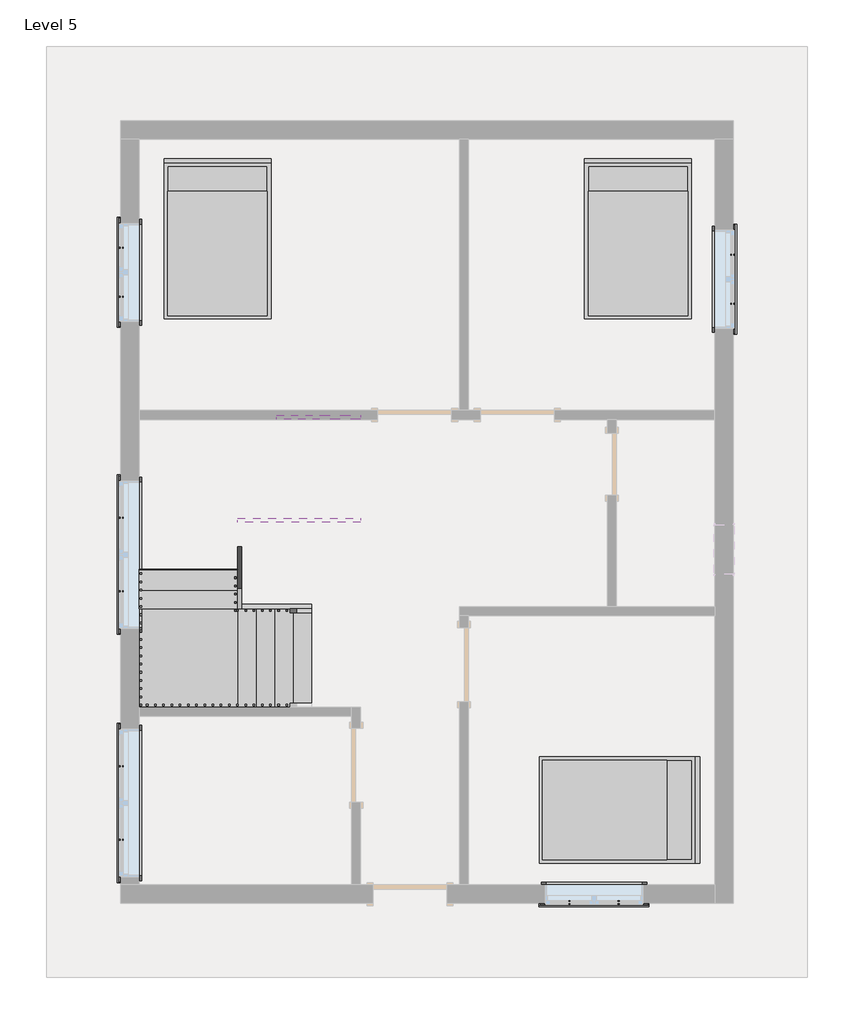
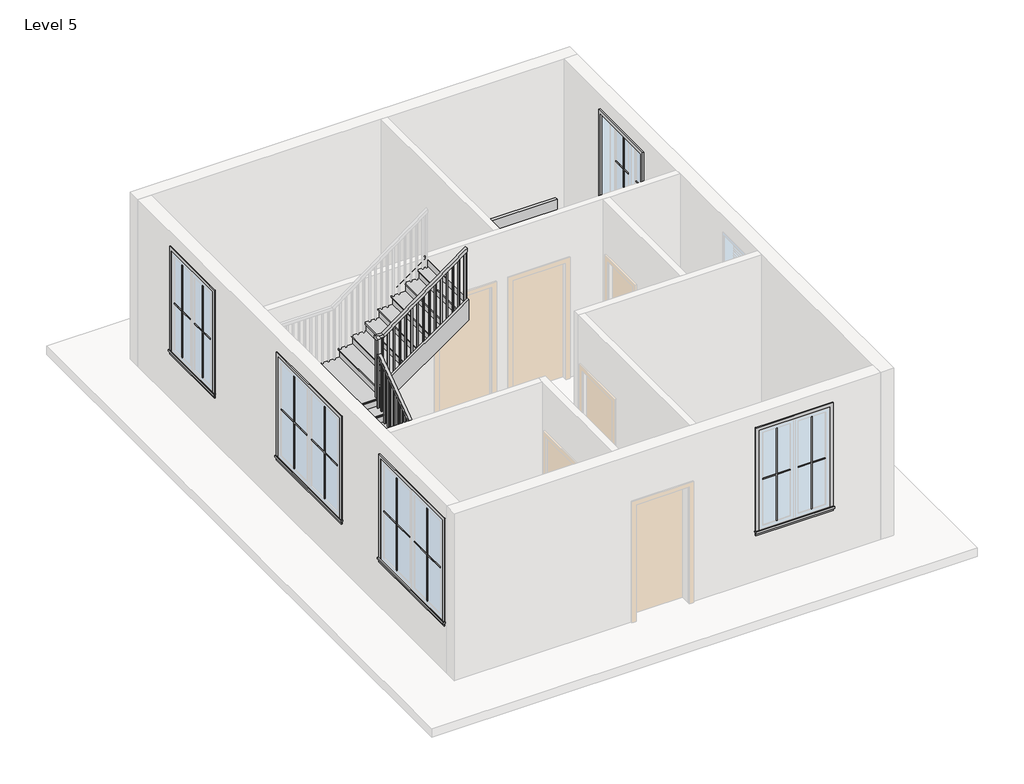
# One storey, part 3 of 3: 20 proxies, 5 members, 3 furniture elements, 1 railing, 1 stair flight.
"""IFC4 building model written with IfcOpenShell, lengths in millimetres."""

from ifc_helpers import new_model, si_unit, frame, origin, place, context, project, spatial, polyline, outline, extrude, faceted_brep, transform, mapped, element, save
from components import muntin_pattern_2x2_muntin_pattern_2x2_0a037076, muntin_pattern_2x2_muntin_pattern_2x2_e6f69628, muntin_pattern_2x2_muntin_pattern_2x2_2b4d9f72, muntin_pattern_2x2_muntin_pattern_2x2_ef995ed3, trim_window_exterior_flat_with_sill_b601e94a, trim_window_exterior_flat_with_sill_b7e4d11c, trim_window_interior_flat_picture_frame_bfefb25c, trim_window_interior_flat_picture_frame_936b8d2a, bed_17739_bed_17739_15c61121, stair_flight_d9589ae6

model = new_model("IFC4")

# Units and contexts
model_context = context("Model", 3, world=origin())
ifc_project = project(units=[si_unit("LENGTHUNIT", "METRE", prefix="MILLI")], contexts=[model_context])

# Site, building, storey
site = spatial("IfcSite", under=ifc_project)
building = spatial("IfcBuilding", under=site)
storey = spatial("IfcBuildingStorey", under=building, Name="Level 5", Elevation=12649.2)

# Proxies
placement = place(None, origin())
muntin_pattern_2x2_muntin_pattern_2x2_shape = muntin_pattern_2x2_muntin_pattern_2x2_0a037076(model_context)
element("IfcBuildingElementProxy", 1, Name="Muntin Pattern_2x2 : Muntin Pattern_2x2", ObjectType="Muntin Pattern_2x2 : Muntin Pattern_2x2", at=placement, inside=storey, context=model_context, shape_type="MappedRepresentation", body=[
    mapped(muntin_pattern_2x2_muntin_pattern_2x2_shape, transform((-5035.7855391, -4380.9248761, 13633.45), x_axis=(0.0, 1.0, 0.0), y_axis=(-1.0, 0.0, 0.0), z_axis=(0.0, 0.0, 1.0))),
])
element("IfcBuildingElementProxy", 2, Name="Muntin Pattern_2x2 : Muntin Pattern_2x2", ObjectType="Muntin Pattern_2x2 : Muntin Pattern_2x2", at=placement, inside=storey, context=model_context, shape_type="MappedRepresentation", body=[
    mapped(muntin_pattern_2x2_muntin_pattern_2x2_shape, transform((-5035.7855391, -1310.6998761, 13633.45), x_axis=(0.0, 1.0, 0.0), y_axis=(-1.0, 0.0, 0.0), z_axis=(0.0, 0.0, 1.0))),
])
muntin_pattern_2x2_muntin_pattern_2x2_2_shape = muntin_pattern_2x2_muntin_pattern_2x2_e6f69628(model_context)
element("IfcBuildingElementProxy", 3, Name="Muntin Pattern_2x2 : Muntin Pattern_2x2", ObjectType="Muntin Pattern_2x2 : Muntin Pattern_2x2", at=placement, inside=storey, context=model_context, shape_type="MappedRepresentation", body=[
    mapped(muntin_pattern_2x2_muntin_pattern_2x2_2_shape, transform((-5035.7855391, -3469.6998761, 13633.45), x_axis=(0.0, -1.0, 0.0), y_axis=(1.0, 0.0, 0.0), z_axis=(0.0, 0.0, 1.0))),
])
element("IfcBuildingElementProxy", 4, Name="Muntin Pattern_2x2 : Muntin Pattern_2x2", ObjectType="Muntin Pattern_2x2 : Muntin Pattern_2x2", at=placement, inside=storey, context=model_context, shape_type="MappedRepresentation", body=[
    mapped(muntin_pattern_2x2_muntin_pattern_2x2_2_shape, transform((-5035.7855391, -399.4748761, 13633.45), x_axis=(0.0, -1.0, 0.0), y_axis=(1.0, 0.0, 0.0), z_axis=(0.0, 0.0, 1.0))),
])
muntin_pattern_2x2_muntin_pattern_2x2_3_shape = muntin_pattern_2x2_muntin_pattern_2x2_2b4d9f72(model_context)
element("IfcBuildingElementProxy", 5, Name="Muntin Pattern_2x2 : Muntin Pattern_2x2", ObjectType="Muntin Pattern_2x2 : Muntin Pattern_2x2", at=placement, inside=storey, context=model_context, shape_type="MappedRepresentation", body=[
    mapped(muntin_pattern_2x2_muntin_pattern_2x2_3_shape, transform((1115.7769609, -5157.2123761, 13633.45), x_axis=(-1.0, 0.0, 0.0), y_axis=(0.0, -1.0, 0.0), z_axis=(0.0, 0.0, 1.0))),
])
element("IfcBuildingElementProxy", 6, Name="Muntin Pattern_2x2 : Muntin Pattern_2x2", ObjectType="Muntin Pattern_2x2 : Muntin Pattern_2x2", at=placement, inside=storey, context=model_context, shape_type="MappedRepresentation", body=[
    mapped(muntin_pattern_2x2_muntin_pattern_2x2_3_shape, transform((2527.0644609, 2851.7251239, 13633.45), x_axis=(0.0, -1.0, 0.0), y_axis=(1.0, 0.0, 0.0), z_axis=(0.0, 0.0, 1.0))),
])
element("IfcBuildingElementProxy", 7, Name="Muntin Pattern_2x2 : Muntin Pattern_2x2", ObjectType="Muntin Pattern_2x2 : Muntin Pattern_2x2", at=placement, inside=storey, context=model_context, shape_type="MappedRepresentation", body=[
    mapped(muntin_pattern_2x2_muntin_pattern_2x2_3_shape, transform((-5035.7855391, 2331.0251239, 13633.45), x_axis=(0.0, 1.0, 0.0), y_axis=(-1.0, 0.0, 0.0), z_axis=(0.0, 0.0, 1.0))),
])
muntin_pattern_2x2_muntin_pattern_2x2_4_shape = muntin_pattern_2x2_muntin_pattern_2x2_ef995ed3(model_context)
element("IfcBuildingElementProxy", 8, Name="Muntin Pattern_2x2 : Muntin Pattern_2x2", ObjectType="Muntin Pattern_2x2 : Muntin Pattern_2x2", at=placement, inside=storey, context=model_context, shape_type="MappedRepresentation", body=[
    mapped(muntin_pattern_2x2_muntin_pattern_2x2_4_shape, transform((509.3519609, -5157.2123761, 13633.45), x_axis=(1.0, 0.0, 0.0), y_axis=(0.0, 1.0, 0.0), z_axis=(0.0, 0.0, 1.0))),
])
element("IfcBuildingElementProxy", 9, Name="Muntin Pattern_2x2 : Muntin Pattern_2x2", ObjectType="Muntin Pattern_2x2 : Muntin Pattern_2x2", at=placement, inside=storey, context=model_context, shape_type="MappedRepresentation", body=[
    mapped(muntin_pattern_2x2_muntin_pattern_2x2_4_shape, transform((2527.0644609, 2245.3001239, 13633.45), x_axis=(0.0, 1.0, 0.0), y_axis=(-1.0, 0.0, 0.0), z_axis=(0.0, 0.0, 1.0))),
])
element("IfcBuildingElementProxy", 10, Name="Muntin Pattern_2x2 : Muntin Pattern_2x2", ObjectType="Muntin Pattern_2x2 : Muntin Pattern_2x2", at=placement, inside=storey, context=model_context, shape_type="MappedRepresentation", body=[
    mapped(muntin_pattern_2x2_muntin_pattern_2x2_4_shape, transform((-5035.7855391, 2937.4501239, 13633.45), x_axis=(0.0, -1.0, 0.0), y_axis=(1.0, 0.0, 0.0), z_axis=(0.0, 0.0, 1.0))),
])
trim_window_exterior_flat_with_sill_shape = trim_window_exterior_flat_with_sill_b601e94a(model_context)
element("IfcBuildingElementProxy", 11, Name="Trim-Window-Exterior-Flat : with Sill", ObjectType="Trim-Window-Exterior-Flat : with Sill", at=placement, inside=storey, context=model_context, shape_type="MappedRepresentation", body=[
    mapped(trim_window_exterior_flat_with_sill_shape, transform((-5045.3105391, -3925.3123761, 15392.4), x_axis=(0.0, -1.0, 0.0), y_axis=(0.0, 0.0, 1.0), z_axis=(-1.0, 0.0, 0.0))),
])
element("IfcBuildingElementProxy", 12, Name="Trim-Window-Exterior-Flat : with Sill", ObjectType="Trim-Window-Exterior-Flat : with Sill", at=placement, inside=storey, context=model_context, shape_type="MappedRepresentation", body=[
    mapped(trim_window_exterior_flat_with_sill_shape, transform((-5045.3105391, -855.0873761, 15392.4), x_axis=(0.0, -1.0, 0.0), y_axis=(0.0, 0.0, 1.0), z_axis=(-1.0, 0.0, 0.0))),
])
trim_window_exterior_flat_with_sill_2_shape = trim_window_exterior_flat_with_sill_b7e4d11c(model_context)
element("IfcBuildingElementProxy", 13, Name="Trim-Window-Exterior-Flat : with Sill", ObjectType="Trim-Window-Exterior-Flat : with Sill", at=placement, inside=storey, context=model_context, shape_type="MappedRepresentation", body=[
    mapped(trim_window_exterior_flat_with_sill_2_shape, transform((812.5644609, -5166.7373761, 15392.4), x_axis=(1.0, 0.0, 0.0), y_axis=(0.0, 0.0, 1.0), z_axis=(0.0, -1.0, 0.0))),
])
element("IfcBuildingElementProxy", 14, Name="Trim-Window-Exterior-Flat : with Sill", ObjectType="Trim-Window-Exterior-Flat : with Sill", at=placement, inside=storey, context=model_context, shape_type="MappedRepresentation", body=[
    mapped(trim_window_exterior_flat_with_sill_2_shape, transform((2536.5894609, 2548.5126239, 15392.4), x_axis=(0.0, 1.0, 0.0), y_axis=(0.0, 0.0, 1.0), z_axis=(1.0, 0.0, 0.0))),
])
element("IfcBuildingElementProxy", 15, Name="Trim-Window-Exterior-Flat : with Sill", ObjectType="Trim-Window-Exterior-Flat : with Sill", at=placement, inside=storey, context=model_context, shape_type="MappedRepresentation", body=[
    mapped(trim_window_exterior_flat_with_sill_2_shape, transform((-5045.3105391, 2634.2376239, 15392.4), x_axis=(0.0, -1.0, 0.0), y_axis=(0.0, 0.0, 1.0), z_axis=(-1.0, 0.0, 0.0))),
])
trim_window_interior_flat_picture_frame_shape = trim_window_interior_flat_picture_frame_bfefb25c(model_context)
element("IfcBuildingElementProxy", 16, Name="Trim-Window-Interior-Flat : Picture Frame", ObjectType="Trim-Window-Interior-Flat : Picture Frame", at=placement, inside=storey, context=model_context, shape_type="MappedRepresentation", body=[
    mapped(trim_window_interior_flat_picture_frame_shape, transform((-4816.7105391, -3925.3123761, 15392.4), x_axis=(0.0, 1.0, 0.0), y_axis=(0.0, 0.0, 1.0), z_axis=(1.0, 0.0, 0.0))),
])
element("IfcBuildingElementProxy", 17, Name="Trim-Window-Interior-Flat : Picture Frame", ObjectType="Trim-Window-Interior-Flat : Picture Frame", at=placement, inside=storey, context=model_context, shape_type="MappedRepresentation", body=[
    mapped(trim_window_interior_flat_picture_frame_shape, transform((-4816.7105391, -855.0873761, 15392.4), x_axis=(0.0, 1.0, 0.0), y_axis=(0.0, 0.0, 1.0), z_axis=(1.0, 0.0, 0.0))),
])
trim_window_interior_flat_picture_frame_2_shape = trim_window_interior_flat_picture_frame_936b8d2a(model_context)
element("IfcBuildingElementProxy", 18, Name="Trim-Window-Interior-Flat : Picture Frame", ObjectType="Trim-Window-Interior-Flat : Picture Frame", at=placement, inside=storey, context=model_context, shape_type="MappedRepresentation", body=[
    mapped(trim_window_interior_flat_picture_frame_2_shape, transform((812.5644609, -4938.1373761, 15392.4), x_axis=(-1.0, 0.0, 0.0), y_axis=(0.0, 0.0, 1.0), z_axis=(0.0, 1.0, 0.0))),
])
element("IfcBuildingElementProxy", 19, Name="Trim-Window-Interior-Flat : Picture Frame", ObjectType="Trim-Window-Interior-Flat : Picture Frame", at=placement, inside=storey, context=model_context, shape_type="MappedRepresentation", body=[
    mapped(trim_window_interior_flat_picture_frame_2_shape, transform((2307.9894609, 2548.5126239, 15392.4), x_axis=(0.0, -1.0, 0.0), y_axis=(0.0, 0.0, 1.0), z_axis=(-1.0, 0.0, 0.0))),
])
element("IfcBuildingElementProxy", 20, Name="Trim-Window-Interior-Flat : Picture Frame", ObjectType="Trim-Window-Interior-Flat : Picture Frame", at=placement, inside=storey, context=model_context, shape_type="MappedRepresentation", body=[
    mapped(trim_window_interior_flat_picture_frame_2_shape, transform((-4816.7105391, 2634.2376239, 15392.4), x_axis=(0.0, 1.0, 0.0), y_axis=(0.0, 0.0, 1.0), z_axis=(1.0, 0.0, 0.0))),
])

# Furniture
bed_17739_bed_17739_shape = bed_17739_bed_17739_15c61121(model_context)
element("IfcFurniture", 21, ObjectType="Bed_17739 : Bed_17739", at=placement, inside=storey, context=model_context, shape_type="MappedRepresentation", body=[
    mapped(bed_17739_bed_17739_shape, transform((-3845.1605391, 3024.7626239, 12649.2), x_axis=(1.0, 0.0, 0.0), y_axis=(0.0, 1.0, 0.0), z_axis=(0.0, 0.0, 1.0))),
])
element("IfcFurniture", 22, ObjectType="Bed_17739 : Bed_17739", at=placement, inside=storey, context=model_context, shape_type="MappedRepresentation", body=[
    mapped(bed_17739_bed_17739_shape, transform((1355.4894609, 3024.7626239, 12649.2), x_axis=(1.0, 0.0, 0.0), y_axis=(0.0, 1.0, 0.0), z_axis=(0.0, 0.0, 1.0))),
])
element("IfcFurniture", 23, ObjectType="Bed_17739 : Bed_17739", at=placement, inside=storey, context=model_context, shape_type="MappedRepresentation", body=[
    mapped(bed_17739_bed_17739_shape, transform((1101.4894609, -4011.0373761, 12649.2), x_axis=(0.0, -1.0, 0.0), y_axis=(1.0, 0.0, 0.0), z_axis=(0.0, 0.0, 1.0))),
])

# Members
element("IfcMember", 24, ObjectType="Stringer - 2\" Width", at=placement, inside=storey, context=model_context, shape_type="SweptSolid", body=[
    extrude(outline(polyline([(12649.2, -2683.1105391), (12799.7087903, -2683.1105391), (12799.7087903, -3112.2707489), (12649.2, -2897.7957228), (12649.2, -2683.1105391)])), frame((0.0, -2791.8373761, 0.0), z_axis=(0.0, 1.0, 0.0), x_axis=(0.0, 0.0, 1.0)), (0.0, 0.0, 1.0), 50.8),
])
element("IfcMember", 25, ObjectType="Stringer - 2\" Width", at=placement, inside=storey, context=model_context, shape_type="SweptSolid", body=[
    extrude(outline(polyline([(14976.6856495, -2580.7583047), (15332.6489938, -2073.5105391), (15705.0117181, -2073.5105391), (14976.6856495, -3111.3751869), (14976.6856495, -2580.7583047)])), frame((0.0, 814.9626239, 0.0), z_axis=(0.0, 1.0, 0.0), x_axis=(0.0, 0.0, 1.0)), (0.0, 0.0, 1.0), 50.8),
])
element("IfcMember", 26, ObjectType="Stringer - 2\" Width", at=placement, inside=storey, context=model_context, shape_type="SweptSolid", body=[
    extrude(outline(polyline([(12649.2, -2683.1105391), (12870.906455, -2683.1105391), (13476.9415427, -3546.7105391), (13104.5788184, -3546.7105391), (12649.2, -2897.7957228), (12649.2, -2683.1105391)])), frame((0.0, -1521.8373761, 0.0), z_axis=(0.0, 1.0, 0.0), x_axis=(0.0, 0.0, 1.0)), (0.0, 0.0, 1.0), 50.8),
])
element("IfcMember", 27, ObjectType="Stringer - 2\" Width", at=placement, inside=storey, context=model_context, shape_type="SweptSolid", body=[
    extrude(outline(polyline([(-1521.8373761, 13299.5564629), (-1521.8373761, 13674.7327137), (-455.0373761, 14440.3786467), (-455.0373761, 14065.2023959), (-1521.8373761, 13299.5564629)])), frame((-3597.5105391, 0.0, 0.0), z_axis=(1.0, 0.0, 0.0), x_axis=(0.0, 1.0, 0.0)), (0.0, 0.0, 1.0), 50.8),
])
element("IfcMember", 28, ObjectType="Stringer - 2\" Width", at=placement, inside=storey, context=model_context, shape_type="SweptSolid", body=[
    extrude(outline(polyline([(14635.5380339, -3597.5105391), (14263.1753096, -3597.5105391), (15332.6489938, -2073.5105391), (15705.0117181, -2073.5105391), (14635.5380339, -3597.5105391)])), frame((0.0, -455.0373761, 0.0), z_axis=(0.0, 1.0, 0.0), x_axis=(0.0, 0.0, 1.0)), (0.0, 0.0, 1.0), 50.8),
])

# Railing
element("IfcRailing", 29, ObjectType="Handrail - Rectangular", at=placement, inside=storey, context=model_context, shape_type="SolidModel", body=[
    faceted_brep([(-2683.1105391, -1572.6373761, 13724.0210526), (-2683.1105391, -1572.6373761, 13661.9605986), (-2683.1105391, -1521.8373761, 13661.9605986), (-2683.1105391, -1521.8373761, 13724.0210526), (-3521.3105391, -1572.6373761, 14312.2315789), (-3572.1105391, -1572.6373761, 14285.8202477), (-3572.1105391, -1521.8373761, 14285.8202477), (-3521.3105391, -1521.8373761, 14312.2315789), (-3521.3105391, -1572.6373761, 14580.815311), (-3572.1105391, -1572.6373761, 14530.015311), (-3572.1105391, -1521.8373761, 14530.015311), (-3521.3105391, -1521.8373761, 14580.815311), (-3648.3105391, -1572.6373761, 14580.815311), (-3648.3105391, -1572.6373761, 14530.015311), (-3597.5105391, -1521.8373761, 14530.015311), (-3597.5105391, -1521.8373761, 14580.815311), (-3648.3105391, -1445.6373761, 14580.815311), (-3648.3105391, -1429.2944467, 14530.015311), (-3597.5105391, -1429.2944467, 14530.015311), (-3597.5105391, -1445.6373761, 14580.815311), (-3648.3105391, -480.4373761, 15273.5425837), (-3648.3105391, -429.6373761, 15247.4725387), (-3597.5105391, -429.6373761, 15247.4725387), (-3597.5105391, -480.4373761, 15273.5425837), (-3648.3105391, -480.4373761, 15544.8), (-3648.3105391, -429.6373761, 15494.0), (-3597.5105391, -429.6373761, 15494.0), (-3597.5105391, -480.4373761, 15544.8), (-3648.3105391, -353.4373761, 15544.8), (-3648.3105391, -353.4373761, 15494.0), (-3597.5105391, -404.2373761, 15494.0), (-3597.5105391, -404.2373761, 15544.8), (-3521.3105391, -353.4373761, 15544.8), (-3504.6160355, -353.4373761, 15494.0), (-3504.6160355, -404.2373761, 15494.0), (-3521.3105391, -404.2373761, 15544.8), (-2073.5105391, -353.4373761, 16611.6), (-2073.5105391, -404.2373761, 16611.6), (-2073.5105391, -404.2373761, 16548.4987868), (-2073.5105391, -353.4373761, 16548.4987868)], [[[0, 1, 2, 3]], [[1, 0, 4, 5]], [[2, 1, 5, 6]], [[3, 2, 6, 7]], [[0, 3, 7, 4]], [[5, 4, 8, 9]], [[6, 5, 9, 10]], [[7, 6, 10, 11]], [[4, 7, 11, 8]], [[9, 8, 12, 13]], [[10, 9, 13, 14]], [[11, 10, 14, 15]], [[8, 11, 15, 12]], [[13, 12, 16, 17]], [[14, 13, 17, 18]], [[15, 14, 18, 19]], [[12, 15, 19, 16]], [[17, 16, 20, 21]], [[18, 17, 21, 22]], [[19, 18, 22, 23]], [[16, 19, 23, 20]], [[21, 20, 24, 25]], [[22, 21, 25, 26]], [[23, 22, 26, 27]], [[20, 23, 27, 24]], [[25, 24, 28, 29]], [[26, 25, 29, 30]], [[27, 26, 30, 31]], [[24, 27, 31, 28]], [[29, 28, 32, 33]], [[30, 29, 33, 34]], [[31, 30, 34, 35]], [[28, 31, 35, 32]], [[36, 37, 38, 39]], [[33, 32, 36, 39]], [[34, 33, 39, 38]], [[35, 34, 38, 37]], [[32, 35, 37, 36]]]),
    extrude(outline(polyline([(16536.8014184, -2089.3855391), (16522.7645763, -2108.4355391), (15536.7789474, -2108.4355391), (15536.7789474, -2089.3855391), (16536.8014184, -2089.3855391)])), frame((0.0, -388.3623761, 0.0), z_axis=(0.0, 1.0, 0.0), x_axis=(0.0, 0.0, 1.0)), (0.0, 0.0, 1.0), 19.05),
    extrude(outline(polyline([(16461.9382605, -2190.9855391), (16447.9014184, -2210.0355391), (15536.7789474, -2210.0355391), (15536.7789474, -2190.9855391), (16461.9382605, -2190.9855391)])), frame((0.0, -388.3623761, 0.0), z_axis=(0.0, 1.0, 0.0), x_axis=(0.0, 0.0, 1.0)), (0.0, 0.0, 1.0), 19.05),
    extrude(outline(polyline([(16387.0751026, -2292.5855391), (16373.0382605, -2311.6355391), (15376.3578947, -2311.6355391), (15376.3578947, -2292.5855391), (16387.0751026, -2292.5855391)])), frame((0.0, -388.3623761, 0.0), z_axis=(0.0, 1.0, 0.0), x_axis=(0.0, 0.0, 1.0)), (0.0, 0.0, 1.0), 19.05),
    extrude(outline(polyline([(16312.2119447, -2394.1855391), (16298.1751026, -2413.2355391), (15376.3578947, -2413.2355391), (15376.3578947, -2394.1855391), (16312.2119447, -2394.1855391)])), frame((0.0, -388.3623761, 0.0), z_axis=(0.0, 1.0, 0.0), x_axis=(0.0, 0.0, 1.0)), (0.0, 0.0, 1.0), 19.05),
    extrude(outline(polyline([(16237.3487868, -2495.7855391), (16223.3119447, -2514.8355391), (15215.9368421, -2514.8355391), (15215.9368421, -2495.7855391), (16237.3487868, -2495.7855391)])), frame((0.0, -388.3623761, 0.0), z_axis=(0.0, 1.0, 0.0), x_axis=(0.0, 0.0, 1.0)), (0.0, 0.0, 1.0), 19.05),
    extrude(outline(polyline([(16162.4856289, -2597.3855391), (16148.4487868, -2616.4355391), (15215.9368421, -2616.4355391), (15215.9368421, -2597.3855391), (16162.4856289, -2597.3855391)])), frame((0.0, -388.3623761, 0.0), z_axis=(0.0, 1.0, 0.0), x_axis=(0.0, 0.0, 1.0)), (0.0, 0.0, 1.0), 19.05),
    extrude(outline(polyline([(16087.622471, -2698.9855391), (16073.5856289, -2718.0355391), (15055.5157895, -2718.0355391), (15055.5157895, -2698.9855391), (16087.622471, -2698.9855391)])), frame((0.0, -388.3623761, 0.0), z_axis=(0.0, 1.0, 0.0), x_axis=(0.0, 0.0, 1.0)), (0.0, 0.0, 1.0), 19.05),
    extrude(outline(polyline([(16012.7593132, -2800.5855391), (15998.722471, -2819.6355391), (15055.5157895, -2819.6355391), (15055.5157895, -2800.5855391), (16012.7593132, -2800.5855391)])), frame((0.0, -388.3623761, 0.0), z_axis=(0.0, 1.0, 0.0), x_axis=(0.0, 0.0, 1.0)), (0.0, 0.0, 1.0), 19.05),
    extrude(outline(polyline([(15937.8961553, -2902.1855391), (15923.8593132, -2921.2355391), (15055.5157895, -2921.2355391), (15055.5157895, -2902.1855391), (15937.8961553, -2902.1855391)])), frame((0.0, -388.3623761, 0.0), z_axis=(0.0, 1.0, 0.0), x_axis=(0.0, 0.0, 1.0)), (0.0, 0.0, 1.0), 19.05),
    extrude(outline(polyline([(15863.0329974, -3003.7855391), (15848.9961553, -3022.8355391), (14895.0947368, -3022.8355391), (14895.0947368, -3003.7855391), (15863.0329974, -3003.7855391)])), frame((0.0, -388.3623761, 0.0), z_axis=(0.0, 1.0, 0.0), x_axis=(0.0, 0.0, 1.0)), (0.0, 0.0, 1.0), 19.05),
    extrude(outline(polyline([(15788.1698395, -3105.3855391), (15774.1329974, -3124.4355391), (14895.0947368, -3124.4355391), (14895.0947368, -3105.3855391), (15788.1698395, -3105.3855391)])), frame((0.0, -388.3623761, 0.0), z_axis=(0.0, 1.0, 0.0), x_axis=(0.0, 0.0, 1.0)), (0.0, 0.0, 1.0), 19.05),
    extrude(outline(polyline([(15713.3066816, -3206.9855391), (15699.2698395, -3226.0355391), (14734.6736842, -3226.0355391), (14734.6736842, -3206.9855391), (15713.3066816, -3206.9855391)])), frame((0.0, -388.3623761, 0.0), z_axis=(0.0, 1.0, 0.0), x_axis=(0.0, 0.0, 1.0)), (0.0, 0.0, 1.0), 19.05),
    extrude(outline(polyline([(15638.4435237, -3308.5855391), (15624.4066816, -3327.6355391), (14734.6736842, -3327.6355391), (14734.6736842, -3308.5855391), (15638.4435237, -3308.5855391)])), frame((0.0, -388.3623761, 0.0), z_axis=(0.0, 1.0, 0.0), x_axis=(0.0, 0.0, 1.0)), (0.0, 0.0, 1.0), 19.05),
    extrude(outline(polyline([(15563.5803658, -3410.1855391), (15549.5435237, -3429.2355391), (14574.2526316, -3429.2355391), (14574.2526316, -3410.1855391), (15563.5803658, -3410.1855391)])), frame((0.0, -388.3623761, 0.0), z_axis=(0.0, 1.0, 0.0), x_axis=(0.0, 0.0, 1.0)), (0.0, 0.0, 1.0), 19.05),
    extrude(outline(polyline([(15488.7172079, -3511.7855391), (15474.6803658, -3530.8355391), (14574.2526316, -3530.8355391), (14574.2526316, -3511.7855391), (15488.7172079, -3511.7855391)])), frame((0.0, -388.3623761, 0.0), z_axis=(0.0, 1.0, 0.0), x_axis=(0.0, 0.0, 1.0)), (0.0, 0.0, 1.0), 19.05),
    extrude(outline(polyline([(-3613.3855391, -439.1623761), (-3632.4355391, -439.1623761), (-3632.4355391, -420.1123761), (-3613.3855391, -420.1123761), (-3613.3855391, -439.1623761)])), frame((0.0, 0.0, 14253.4105263), z_axis=(0.0, 0.0, 1.0), x_axis=(1.0, 0.0, 0.0)), (0.0, 0.0, 1.0), 1240.5894737),
    extrude(outline(polyline([(-540.7623761, 15167.7177541), (-521.7123761, 15181.3900029), (-521.7123761, 14253.4105263), (-540.7623761, 14253.4105263), (-540.7623761, 15167.7177541)])), frame((-3632.4355391, 0.0, 0.0), z_axis=(1.0, 0.0, 0.0), x_axis=(0.0, 1.0, 0.0)), (0.0, 0.0, 1.0), 19.05),
    extrude(outline(polyline([(-642.3623761, 15094.7990938), (-623.3123761, 15108.4713426), (-623.3123761, 14092.9894737), (-642.3623761, 14092.9894737), (-642.3623761, 15094.7990938)])), frame((-3632.4355391, 0.0, 0.0), z_axis=(1.0, 0.0, 0.0), x_axis=(0.0, 1.0, 0.0)), (0.0, 0.0, 1.0), 19.05),
    extrude(outline(polyline([(-743.9623761, 15021.8804335), (-724.9123761, 15035.5526823), (-724.9123761, 14092.9894737), (-743.9623761, 14092.9894737), (-743.9623761, 15021.8804335)])), frame((-3632.4355391, 0.0, 0.0), z_axis=(1.0, 0.0, 0.0), x_axis=(0.0, 1.0, 0.0)), (0.0, 0.0, 1.0), 19.05),
    extrude(outline(polyline([(-845.5623761, 14948.9617732), (-826.5123761, 14962.634022), (-826.5123761, 14092.9894737), (-845.5623761, 14092.9894737), (-845.5623761, 14948.9617732)])), frame((-3632.4355391, 0.0, 0.0), z_axis=(1.0, 0.0, 0.0), x_axis=(0.0, 1.0, 0.0)), (0.0, 0.0, 1.0), 19.05),
    extrude(outline(polyline([(-947.1623761, 14876.0431129), (-928.1123761, 14889.7153617), (-928.1123761, 13932.5684211), (-947.1623761, 13932.5684211), (-947.1623761, 14876.0431129)])), frame((-3632.4355391, 0.0, 0.0), z_axis=(1.0, 0.0, 0.0), x_axis=(0.0, 1.0, 0.0)), (0.0, 0.0, 1.0), 19.05),
    extrude(outline(polyline([(-1048.7623761, 14803.1244526), (-1029.7123761, 14816.7967014), (-1029.7123761, 13932.5684211), (-1048.7623761, 13932.5684211), (-1048.7623761, 14803.1244526)])), frame((-3632.4355391, 0.0, 0.0), z_axis=(1.0, 0.0, 0.0), x_axis=(0.0, 1.0, 0.0)), (0.0, 0.0, 1.0), 19.05),
    extrude(outline(polyline([(-1150.3623761, 14730.2057923), (-1131.3123761, 14743.8780411), (-1131.3123761, 13772.1473684), (-1150.3623761, 13772.1473684), (-1150.3623761, 14730.2057923)])), frame((-3632.4355391, 0.0, 0.0), z_axis=(1.0, 0.0, 0.0), x_axis=(0.0, 1.0, 0.0)), (0.0, 0.0, 1.0), 19.05),
    extrude(outline(polyline([(-1251.9623761, 14657.287132), (-1232.9123761, 14670.9593808), (-1232.9123761, 13772.1473684), (-1251.9623761, 13772.1473684), (-1251.9623761, 14657.287132)])), frame((-3632.4355391, 0.0, 0.0), z_axis=(1.0, 0.0, 0.0), x_axis=(0.0, 1.0, 0.0)), (0.0, 0.0, 1.0), 19.05),
    extrude(outline(polyline([(-1353.5623761, 14584.3684718), (-1334.5123761, 14598.0407206), (-1334.5123761, 13611.7263158), (-1353.5623761, 13611.7263158), (-1353.5623761, 14584.3684718)])), frame((-3632.4355391, 0.0, 0.0), z_axis=(1.0, 0.0, 0.0), x_axis=(0.0, 1.0, 0.0)), (0.0, 0.0, 1.0), 19.05),
    extrude(outline(polyline([(-1455.1623761, 14511.4498115), (-1436.1123761, 14525.1220603), (-1436.1123761, 13611.7263158), (-1455.1623761, 13611.7263158), (-1455.1623761, 14511.4498115)])), frame((-3632.4355391, 0.0, 0.0), z_axis=(1.0, 0.0, 0.0), x_axis=(0.0, 1.0, 0.0)), (0.0, 0.0, 1.0), 19.05),
    extrude(outline(polyline([(-3587.9855391, -1537.7123761), (-3587.9855391, -1556.7623761), (-3607.0355391, -1556.7623761), (-3607.0355391, -1537.7123761), (-3587.9855391, -1537.7123761)])), frame((0.0, 0.0, 13451.3052632), z_axis=(0.0, 0.0, 1.0), x_axis=(1.0, 0.0, 0.0)), (0.0, 0.0, 1.0), 1078.7100478),
    extrude(outline(polyline([(14225.662353, -3486.3855391), (14239.030774, -3505.4355391), (13290.8842105, -3505.4355391), (13290.8842105, -3486.3855391), (14225.662353, -3486.3855391)])), frame((0.0, -1556.7623761, 0.0), z_axis=(0.0, 1.0, 0.0), x_axis=(0.0, 0.0, 1.0)), (0.0, 0.0, 1.0), 19.05),
    extrude(outline(polyline([(14154.3641074, -3384.7855391), (14167.7325284, -3403.8355391), (13290.8842105, -3403.8355391), (13290.8842105, -3384.7855391), (14154.3641074, -3384.7855391)])), frame((0.0, -1556.7623761, 0.0), z_axis=(0.0, 1.0, 0.0), x_axis=(0.0, 0.0, 1.0)), (0.0, 0.0, 1.0), 19.05),
    extrude(outline(polyline([(14083.0658617, -3283.1855391), (14096.4342828, -3302.2355391), (13130.4631579, -3302.2355391), (13130.4631579, -3283.1855391), (14083.0658617, -3283.1855391)])), frame((0.0, -1556.7623761, 0.0), z_axis=(0.0, 1.0, 0.0), x_axis=(0.0, 0.0, 1.0)), (0.0, 0.0, 1.0), 19.05),
    extrude(outline(polyline([(14011.7676161, -3181.5855391), (14025.1360372, -3200.6355391), (13130.4631579, -3200.6355391), (13130.4631579, -3181.5855391), (14011.7676161, -3181.5855391)])), frame((0.0, -1556.7623761, 0.0), z_axis=(0.0, 1.0, 0.0), x_axis=(0.0, 0.0, 1.0)), (0.0, 0.0, 1.0), 19.05),
    extrude(outline(polyline([(13940.4693705, -3079.9855391), (13953.8377916, -3099.0355391), (12970.0421053, -3099.0355391), (12970.0421053, -3079.9855391), (13940.4693705, -3079.9855391)])), frame((0.0, -1556.7623761, 0.0), z_axis=(0.0, 1.0, 0.0), x_axis=(0.0, 0.0, 1.0)), (0.0, 0.0, 1.0), 19.05),
    extrude(outline(polyline([(13869.1711249, -2978.3855391), (13882.5395459, -2997.4355391), (12970.0421053, -2997.4355391), (12970.0421053, -2978.3855391), (13869.1711249, -2978.3855391)])), frame((0.0, -1556.7623761, 0.0), z_axis=(0.0, 1.0, 0.0), x_axis=(0.0, 0.0, 1.0)), (0.0, 0.0, 1.0), 19.05),
    extrude(outline(polyline([(13797.8728793, -2876.7855391), (13811.2413003, -2895.8355391), (12809.6210526, -2895.8355391), (12809.6210526, -2876.7855391), (13797.8728793, -2876.7855391)])), frame((0.0, -1556.7623761, 0.0), z_axis=(0.0, 1.0, 0.0), x_axis=(0.0, 0.0, 1.0)), (0.0, 0.0, 1.0), 19.05),
    extrude(outline(polyline([(13726.5746337, -2775.1855391), (13739.9430547, -2794.2355391), (12809.6210526, -2794.2355391), (12809.6210526, -2775.1855391), (13726.5746337, -2775.1855391)])), frame((0.0, -1556.7623761, 0.0), z_axis=(0.0, 1.0, 0.0), x_axis=(0.0, 0.0, 1.0)), (0.0, 0.0, 1.0), 19.05),
    extrude(outline(polyline([(-3613.3855391, -388.3623761), (-3632.4355391, -388.3623761), (-3632.4355391, -369.3123761), (-3613.3855391, -369.3123761), (-3613.3855391, -388.3623761)])), frame((0.0, 0.0, 14413.8315789), z_axis=(0.0, 0.0, 1.0), x_axis=(1.0, 0.0, 0.0)), (0.0, 0.0, 1.0), 1080.1684211),
    extrude(outline(polyline([(-3613.3855391, -1537.7123761), (-3613.3855391, -1556.7623761), (-3632.4355391, -1556.7623761), (-3632.4355391, -1537.7123761), (-3613.3855391, -1537.7123761)])), frame((0.0, 0.0, 13451.3052632), z_axis=(0.0, 0.0, 1.0), x_axis=(1.0, 0.0, 0.0)), (0.0, 0.0, 1.0), 1078.7100478),
    extrude(outline(polyline([(16548.4987868, -2073.5105391), (16534.4619447, -2092.5605391), (15536.7789474, -2092.5605391), (15536.7789474, -2073.5105391), (16548.4987868, -2073.5105391)])), frame((0.0, -388.3623761, 0.0), z_axis=(0.0, 1.0, 0.0), x_axis=(0.0, 0.0, 1.0)), (0.0, 0.0, 1.0), 19.05),
    extrude(outline(polyline([(13661.9605986, -2683.1105391), (13675.3290196, -2702.1605391), (12809.6210526, -2702.1605391), (12809.6210526, -2683.1105391), (13661.9605986, -2683.1105391)])), frame((0.0, -1556.7623761, 0.0), z_axis=(0.0, 1.0, 0.0), x_axis=(0.0, 0.0, 1.0)), (0.0, 0.0, 1.0), 19.05),
])

# Stair flight
stair_flight_shape = stair_flight_d9589ae6(model_context)
element("IfcStairFlight", 30, ObjectType="2\" Tread 1\" Nosing 1/4\" Riser", at=placement, inside=storey, context=model_context, shape_type="MappedRepresentation", body=[
    mapped(stair_flight_shape, transform((0.0, 0.0, 0.0), x_axis=(1.0, 0.0, 0.0), y_axis=(0.0, 1.0, 0.0), z_axis=(0.0, 0.0, 1.0))),
])

save(model, "model.ifc")

# Revit data of these elements
# Type "Muntin Pattern_2x2 : Muntin Pattern_2x2"
#   Width [instance default] = 4' - 0"
#   Thickness = 0' - 0 1/2"
#   Height [instance default] = 4' - 0"
#   Distance = 0' - 0 3/4"
#   Interior Material [instance default] = none
#   Exterior Material [instance default] = none
#   Default Elevation = 0
# Type "Trim-Window-Exterior-Flat : with Sill"
#   Trim Width = 0' - 2 1/4"
#   Trim Thickness_Picture Frame = 0' - 1 1/4"
#   Trim Thickness_with Sill = 0' - 0 3/4"
#   Sill Thickness = 0' - 1 1/4"
#   Opening Width [instance default] = 2' - 0"
#   Opening Height [instance default] = 3' - 0"
#   Default Elevation = 4' - 0"
#   Sill = yes
#   Picture Frame = no
#   Trim Material [instance default] = none
# Type "Trim-Window-Interior-Flat : Picture Frame"
#   Trim Thickness_Picture Frame = 0' - 1 1/4"
#   Trim Width = 0' - 2 1/4"
#   Trim Thickness_with Sill = 0' - 0 3/4"
#   Sill Thickness = 0' - 1 1/4"
#   Opening Width [instance default] = 2' - 0"
#   Opening Height [instance default] = 3' - 0"
#   Default Elevation = 4' - 0"
#   Sill = no
#   Picture Frame = yes
#   Trim Material [instance default] = none
# Type "Bed_17739 : Bed_17739"
#   Default Elevation = 0
# Type "Handrail - Rectangular"
#   Assembly Code = "C2010400"
#   built-in parameter 1008612 = 0.0416667 (stored number, unit not read)
#   built-in parameter 1008611 = 0.0416667 (stored number, unit not read)
#   built-in parameter 1008609 = 0.333333 (stored number, unit not read)
#   built-in parameter 1008604 = 0.166667 (stored number, unit not read)
#   built-in parameter 1008603 = 0.166667 (stored number, unit not read)
#   Railing Height = 3' - 0"
#   built-in parameter 1008630 = 2
#   built-in parameter 1008610 = 2
#   built-in parameter 1008618 = Baluster - Square : 3/4"
# Elements 1, 2, 3, 4 (IfcBuildingElementProxy, "Muntin Pattern_2x2 : Muntin Pattern_2x2")
#   Width = 2' - 6 5/8"
#   Height = 5' - 6 1/2"
#   Interior Material = Wood - Stained
#   Exterior Material = Clad - White
#   Phase Created = New Construction
#   Materials on its faces: "Clad - White", "Wood - Stained"
# Elements 5, 6, 7, 8, 9, 10 (IfcBuildingElementProxy, "Muntin Pattern_2x2 : Muntin Pattern_2x2")
#   Width = 1' - 6 5/8"
#   Height = 5' - 6 1/2"
#   Interior Material = Wood - Stained
#   Exterior Material = Clad - White
#   Phase Created = New Construction
#   Materials on its faces: "Clad - White", "Wood - Stained"
# Elements 11, 12 (IfcBuildingElementProxy, "Trim-Window-Exterior-Flat : with Sill")
#   Opening Width = 6' - 0"
#   Opening Height = 6' - 0"
#   Trim Material = Clad - White
#   Phase Created = New Construction
#   Materials on its faces: "Clad - White"
# Elements 13, 14, 15 (IfcBuildingElementProxy, "Trim-Window-Exterior-Flat : with Sill")
#   Opening Width = 4' - 0"
#   Opening Height = 6' - 0"
#   Trim Material = Clad - White
#   Phase Created = New Construction
#   Materials on its faces: "Clad - White"
# Elements 16, 17 (IfcBuildingElementProxy, "Trim-Window-Interior-Flat : Picture Frame")
#   Opening Width = 6' - 0"
#   Opening Height = 6' - 0"
#   Trim Material = Wood - Stained
#   Phase Created = New Construction
#   Materials on its faces: "Wood - Stained"
# Elements 18, 19, 20 (IfcBuildingElementProxy, "Trim-Window-Interior-Flat : Picture Frame")
#   Opening Width = 4' - 0"
#   Opening Height = 6' - 0"
#   Trim Material = Wood - Stained
#   Phase Created = New Construction
#   Materials on its faces: "Wood - Stained"
# Elements 21, 22, 23 (IfcFurniture, "Bed_17739 : Bed_17739")
#   Phase Created = New Construction
#   Materials on its faces: "legs", "sheets", "bed frame", "Blanket"
# Elements 24, 25, 26, 27, 28 (IfcMember, "Stringer - 2\" Width")
#   Phase Created = New Construction
# Element 29 (IfcRailing, "Handrail - Rectangular")
#   Phase Created = New Construction
# Element 30 (IfcStairFlight, "2\" Tread 1\" Nosing 1/4\" Riser")
#   Phase Created = New Construction
# Materials
#   "Clad - White": class "Wood", colour RGB 242 242 238, transparency 0, Cost = 0
#   "Wood - Stained": class "Wood", colour RGB 224 178 126, transparency 0, Cost = 0
#   "legs": colour RGB 90 73 37, transparency 0, Cost = 0
#   "sheets": colour RGB 200 195 176, transparency 0, Cost = 0
#   "bed frame": colour RGB 90 73 37, transparency 0, Cost = 0
#   "Blanket": class "System", colour RGB 59 0 1, transparency 0, Cost = 0
